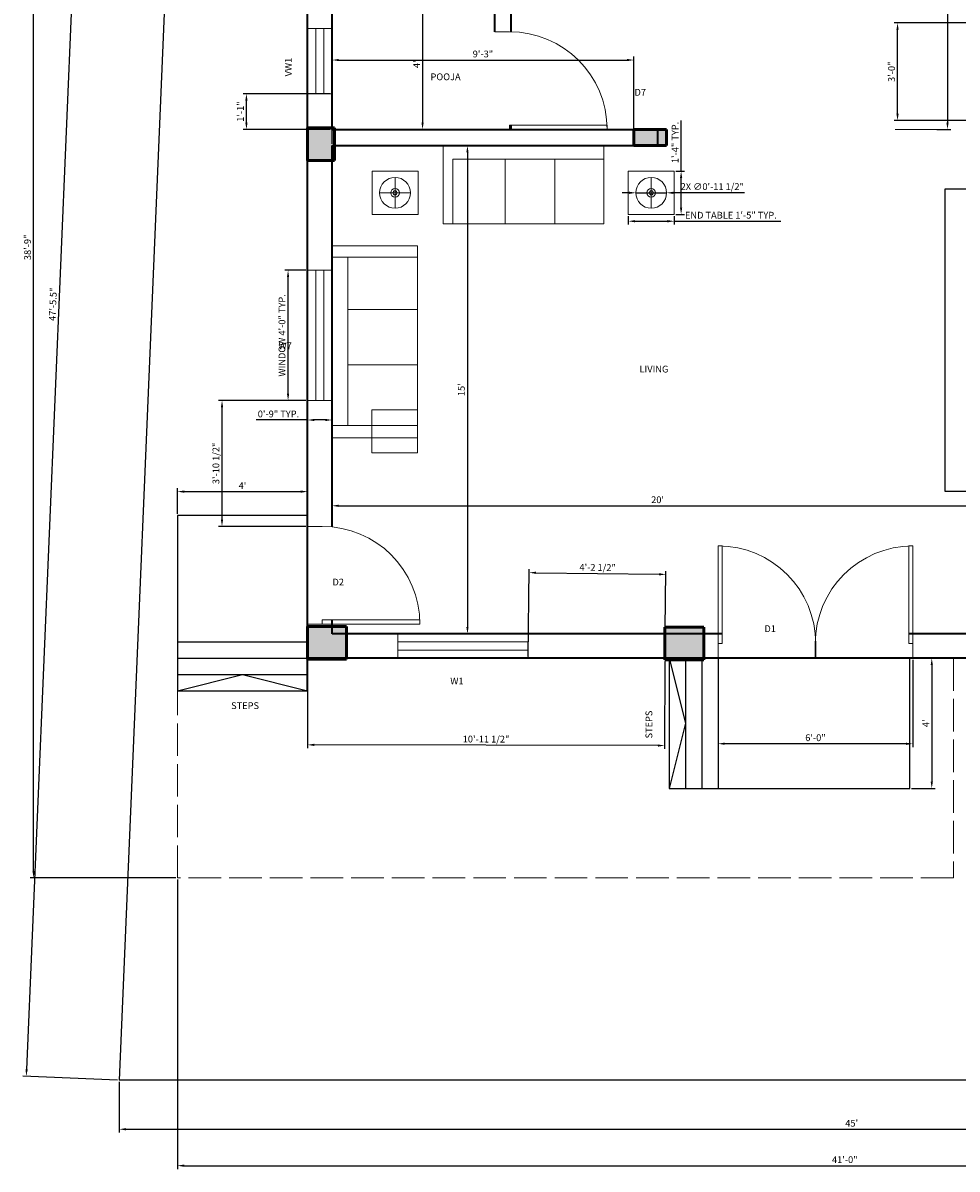
# Model space of a CAD drawing. Units: inches. Extents: x 2470 to 6338, y 1562 to 4199.
# Tile 1 of 5: x 2471 to 2816, y 1562 to 1985. Entities that reach past the tile are written whole.
import ezdxf

# ---------------------------------------------------------------- set-up
doc = ezdxf.new("R2010")
doc.units = ezdxf.units.IN
doc.linetypes.add('ACAD_ISO02W100', pattern=[15, 12, -3])
for name, color, linetype, lineweight in [('A-ANNO-DIMS', 2, 'Continuous', 18), ('A-ANNO-TEXT', 7, 'Continuous', 18), ('A-AREA-IDEN', 7, 'Continuous', 25), ('A-COLS', 1, 'Continuous', 50), ('A-DOOR', 4, 'Continuous', 18), ('A-FLOR-OVHD', 8, 'ACAD_ISO02W100', 18), ('A-FLOR-STRS', 7, 'Continuous', 25), ('A-FURN', 8, 'Continuous', 18), ('A-FURN-FIXD', 8, 'Continuous', 25), ('A-GLAZ', 4, 'Continuous', 18), ('A-WALL', 7, 'Continuous', 35), ('C-PROP', 3, 'Continuous', 25)]:
    doc.layers.add(name, color=color, linetype=linetype, lineweight=lineweight)
doc.styles.get("Standard").update_dxf_attribs({"font": 'arial.ttf'})
doc.dimstyles.new('ISO-25', dxfattribs={"dimtxt": 2.5, "dimasz": 2.5, "dimexe": 1.25, "dimexo": 0.625, "dimtad": 1, "dimdec": 1, "dimlunit": 3, "dimtxsty": 'Standard', "dimcen": 2.5, "dimadec": 0, "dimazin": 0, "dimtfac": 1, "dimtdec": 1, "dimtmove": 0, "dimatfit": 3, "dimfxl": 1, "dimarcsym": 0})

# ---------------------------------------------------------------- blocks, each defined once
blk = doc.blocks.new('*U2')
for p, q in [((0, 0), (0, -6)), ((40, 0), (40, -6))]:
    blk.add_line(p, q)
blk.add_lwpolyline([(0, 0), (0, 40), (1.75, 40), (1.75, 0)], close=True)
blk.add_arc((0, 0), 40, 0, 90)
blk = doc.blocks.new('*D7')
at = {"layer": 'A-ANNO-DIMS', "color": 0, "lineweight": -2, "transparency": 16777216}
for p, q in [((2530.1, 2164.02), (2495.24, 2165.49)), ((2496.38, 2162.94), (2472.59, 1598.93)), ((2506.1, 1595.02), (2471.24, 1596.49))]:
    blk.add_line(p, q, dxfattribs=at)
at = {"layer": 'A-ANNO-DIMS', "color": 0, "lineweight": 100, "transparency": 16777216}
for points in [[(2495.96, 2162.95), (2496.8, 2162.92), (2496.48, 2165.43)], [(2472.17, 1598.95), (2473.01, 1598.92), (2472.48, 1596.43)]]:
    blk.add_solid(points, dxfattribs=at)
at = {"layer": 'Defpoints', "color": 0, "lineweight": 100, "transparency": 16777216}
for p in [(2530.72, 2163.99), (2472.48, 1596.43), (2506.72, 1594.99)]:
    blk.add_point(p, dxfattribs=at)
at = {"layer": 'A-ANNO-DIMS', "color": 0, "transparency": 16777216, "insert": (2482.59, 1881.01), "char_height": 2.5, "attachment_point": 5, "rotation": 87.5847}
blk.add_mtext('47\'-5.5"', dxfattribs=at)
blk = doc.blocks.new('*D10')
at = {"layer": 'A-ANNO-DIMS', "color": 0, "lineweight": -2, "transparency": 16777216}
for p, q in [((2506.72, 1594.37), (2506.72, 1575.62)), ((3046.72, 1594.37), (3046.72, 1575.62)), ((2509.22, 1576.87), (3044.22, 1576.87))]:
    blk.add_line(p, q, dxfattribs=at)
at = {"layer": 'A-ANNO-DIMS', "color": 0, "lineweight": 100, "transparency": 16777216}
for points in [[(2509.22, 1577.29), (2509.22, 1576.46), (2506.72, 1576.87)], [(3044.22, 1577.29), (3044.22, 1576.46), (3046.72, 1576.87)]]:
    blk.add_solid(points, dxfattribs=at)
at = {"layer": 'Defpoints', "color": 0, "lineweight": 100, "transparency": 16777216}
for p in [(2506.72, 1594.99), (3046.72, 1594.99), (3046.72, 1576.87)]:
    blk.add_point(p, dxfattribs=at)
at = {"layer": 'A-ANNO-DIMS', "color": 0, "transparency": 16777216, "insert": (2776.72, 1578.77), "char_height": 2.5, "attachment_point": 5}
blk.add_mtext("45'", dxfattribs=at)
blk = doc.blocks.new('*D13')
at = {"layer": 'A-ANNO-DIMS', "color": 0, "lineweight": -2, "transparency": 16777216}
for p, q in [((2528.17, 1803.76), (2528.17, 1813.21)), ((2576.17, 1803.76), (2576.17, 1813.21)), ((2530.67, 1811.96), (2573.67, 1811.96))]:
    blk.add_line(p, q, dxfattribs=at)
at = {"layer": 'A-ANNO-DIMS', "color": 0, "lineweight": 100, "transparency": 16777216}
for points in [[(2530.67, 1812.38), (2530.67, 1811.55), (2528.17, 1811.96)], [(2573.67, 1812.38), (2573.67, 1811.55), (2576.17, 1811.96)]]:
    blk.add_solid(points, dxfattribs=at)
at = {"layer": 'Defpoints', "color": 0, "lineweight": 100, "transparency": 16777216}
for p in [(2576.17, 1811.96), (2528.17, 1803.13), (2576.17, 1803.13)]:
    blk.add_point(p, dxfattribs=at)
at = {"layer": 'A-ANNO-DIMS', "color": 0, "transparency": 16777216, "insert": (2552.17, 1813.84), "char_height": 2.5, "attachment_point": 5}
blk.add_mtext("4'", dxfattribs=at)
blk = doc.blocks.new('*D14')
at = {"layer": 'A-ANNO-DIMS', "color": 0, "lineweight": -2, "transparency": 16777216}
for p, q in [((2798.79, 1750.53), (2807.48, 1750.53)), ((2806.23, 1748.03), (2806.23, 1705.06)), ((2798.79, 1702.56), (2807.48, 1702.56))]:
    blk.add_line(p, q, dxfattribs=at)
at = {"layer": 'A-ANNO-DIMS', "color": 0, "lineweight": 100, "transparency": 16777216}
for points in [[(2805.82, 1748.03), (2806.65, 1748.03), (2806.23, 1750.53)], [(2805.82, 1705.06), (2806.65, 1705.06), (2806.23, 1702.56)]]:
    blk.add_solid(points, dxfattribs=at)
at = {"layer": 'Defpoints', "color": 0, "lineweight": 100, "transparency": 16777216}
for p in [(2798.17, 1750.53), (2798.17, 1702.56), (2806.23, 1702.56)]:
    blk.add_point(p, dxfattribs=at)
at = {"layer": 'A-ANNO-DIMS', "color": 0, "transparency": 16777216, "insert": (2804.36, 1726.55), "char_height": 2.5, "attachment_point": 5, "rotation": 90}
blk.add_mtext("4'", dxfattribs=at)
blk = doc.blocks.new('*D15')
at = {"layer": 'A-ANNO-DIMS', "color": 0, "lineweight": -2, "transparency": 16777216}
for p, q in [((2585.17, 1813.52), (2585.17, 1805.49)), ((2825.17, 1813.52), (2825.17, 1805.49)), ((2587.67, 1806.74), (2822.67, 1806.74))]:
    blk.add_line(p, q, dxfattribs=at)
at = {"layer": 'A-ANNO-DIMS', "color": 0, "lineweight": 100, "transparency": 16777216}
for points in [[(2587.67, 1807.16), (2587.67, 1806.32), (2585.17, 1806.74)], [(2822.67, 1807.16), (2822.67, 1806.32), (2825.17, 1806.74)]]:
    blk.add_solid(points, dxfattribs=at)
at = {"layer": 'Defpoints', "color": 0, "lineweight": 100, "transparency": 16777216}
for p in [(2585.17, 1814.14), (2825.17, 1814.14), (2825.17, 1806.74)]:
    blk.add_point(p, dxfattribs=at)
at = {"layer": 'A-ANNO-DIMS', "color": 0, "transparency": 16777216, "insert": (2705.17, 1808.64), "char_height": 2.5, "attachment_point": 5}
blk.add_mtext("20'", dxfattribs=at)
blk = doc.blocks.new('*D16')
at = {"layer": 'A-ANNO-DIMS', "color": 0, "lineweight": -2, "transparency": 16777216}
for p, q in [((2621.84, 1939.53), (2636.34, 1939.53)), ((2635.09, 1937.03), (2635.09, 1762.03)), ((2621.84, 1759.53), (2636.34, 1759.53))]:
    blk.add_line(p, q, dxfattribs=at)
at = {"layer": 'A-ANNO-DIMS', "color": 0, "lineweight": 100, "transparency": 16777216}
for points in [[(2634.67, 1937.03), (2635.5, 1937.03), (2635.09, 1939.53)], [(2634.67, 1762.03), (2635.5, 1762.03), (2635.09, 1759.53)]]:
    blk.add_solid(points, dxfattribs=at)
at = {"layer": 'Defpoints', "color": 0, "lineweight": 100, "transparency": 16777216}
for p in [(2621.21, 1939.53), (2621.21, 1759.53), (2635.09, 1759.53)]:
    blk.add_point(p, dxfattribs=at)
at = {"layer": 'A-ANNO-DIMS', "color": 0, "transparency": 16777216, "insert": (2633.18, 1849.53), "char_height": 2.5, "attachment_point": 5, "rotation": 90}
blk.add_mtext("15'", dxfattribs=at)
blk = doc.blocks.new('*D23')
at = {"layer": 'A-ANNO-DIMS', "color": 0, "lineweight": -2, "transparency": 16777216}
for p, q in [((2615.79, 1993.53), (2619.79, 1993.53)), ((2618.54, 1991.03), (2618.54, 1948.03)), ((2615.79, 1945.53), (2619.79, 1945.53))]:
    blk.add_line(p, q, dxfattribs=at)
at = {"layer": 'A-ANNO-DIMS', "color": 0, "lineweight": 100, "transparency": 16777216}
for points in [[(2618.13, 1991.03), (2618.96, 1991.03), (2618.54, 1993.53)], [(2618.13, 1948.03), (2618.96, 1948.03), (2618.54, 1945.53)]]:
    blk.add_solid(points, dxfattribs=at)
at = {"layer": 'Defpoints', "color": 0, "lineweight": 100, "transparency": 16777216}
for p in [(2615.17, 1993.53), (2615.17, 1945.53), (2618.54, 1945.53)]:
    blk.add_point(p, dxfattribs=at)
at = {"layer": 'A-ANNO-DIMS', "color": 0, "transparency": 16777216, "insert": (2616.67, 1969.53), "char_height": 2.5, "attachment_point": 5, "rotation": 90}
blk.add_mtext("4'", dxfattribs=at)
blk = doc.blocks.new('*D28')
at = {"layer": 'A-ANNO-DIMS', "color": 0, "lineweight": -2, "transparency": 16777216}
for p, q in [((2808.15, 2125.53), (2813.28, 2125.53)), ((2812.03, 2123.03), (2812.03, 1948.03)), ((2808.15, 1945.53), (2813.28, 1945.53))]:
    blk.add_line(p, q, dxfattribs=at)
at = {"layer": 'A-ANNO-DIMS', "color": 0, "lineweight": 100, "transparency": 16777216}
for points in [[(2811.62, 2123.03), (2812.45, 2123.03), (2812.03, 2125.53)], [(2811.62, 1948.03), (2812.45, 1948.03), (2812.03, 1945.53)]]:
    blk.add_solid(points, dxfattribs=at)
at = {"layer": 'Defpoints', "color": 0, "lineweight": 100, "transparency": 16777216}
for p in [(2807.53, 2125.53), (2807.53, 1945.53), (2812.03, 1945.53)]:
    blk.add_point(p, dxfattribs=at)
at = {"layer": 'A-ANNO-DIMS', "color": 0, "transparency": 16777216, "insert": (2810.13, 2035.53), "char_height": 2.5, "attachment_point": 5, "rotation": 90}
blk.add_mtext("15'", dxfattribs=at)
blk = doc.blocks.new('WIN-48IN')
for p, q in [((0, 9), (48, 9)), ((0, 0), (0, 9)), ((48, 9), (48, 0)), ((0, 6), (48, 6)), ((48, 3), (0, 3)), ((48, 0), (0, 0))]:
    blk.add_line(p, q)
blk = doc.blocks.new('VENT-WIN-24IN')
for p, q in [((9, 24), (0, 24)), ((0, 24), (0, 0)), ((3, 24), (3, 0)), ((6, 0), (6, 24)), ((9, 0), (9, 24)), ((0, 0), (9, 0))]:
    blk.add_line(p, q)
blk = doc.blocks.new('COL-6X12')
h = blk.add_hatch(color=256)
h.dxf.hatch_style = 1
h.paths.add_polyline_path([(6, 12), (0, 12), (0, 0), (6, 0)])
for p, q in [((6, 12), (0, 12)), ((0, 12), (0, 0)), ((6, 0), (6, 12)), ((0, 0), (6, 0))]:
    blk.add_line(p, q)
blk = doc.blocks.new('COL-10X12')
h = blk.add_hatch(color=256)
h.dxf.hatch_style = 1
h.paths.add_polyline_path([(10, 12), (0, 12), (0, 0), (10, 0)])
for p, q in [((10, 12), (0, 12)), ((0, 12), (0, 0)), ((10, 0), (10, 12)), ((0, 0), (10, 0))]:
    blk.add_line(p, q)
blk = doc.blocks.new('COL-RECT-LARGE')
h = blk.add_hatch(color=256)
h.dxf.hatch_style = 1
h.paths.add_polyline_path([(14.33, 12.11), (10, 12.11), (0, 12.11), (0, 0), (10, 0), (14.33, 0)])
for p, q in [((10, 12.11), (0, 12.11)), ((0, 12.11), (0, 0)), ((10, 12.11), (14.33, 12.11)), ((14.33, 12.11), (14.33, 0)), ((10, 0), (0, 0)), ((14.33, 0), (10, 0))]:
    blk.add_line(p, q)
blk = doc.blocks.new('END-TABLE-LAMP')
for q in [(8.47, 13.6), (2.8, 7.93), (14.14, 7.93), (8.47, 2.26)]:
    blk.add_line((8.47, 7.93), q)
blk.add_lwpolyline([(0, 15.87), (16.95, 15.87), (16.95, 0), (0, 0)], close=True)
for radius in [5.67, 1.6, 0.75]:
    blk.add_circle((8.47, 7.93), radius)
blk = doc.blocks.new('*D38')
at = {"layer": 'A-ANNO-DIMS', "color": 0, "lineweight": -2, "transparency": 16777216}
for p, q in [((2575.54, 1893.57), (2567.72, 1893.57)), ((2568.97, 1848.07), (2568.97, 1891.07)), ((2575.54, 1845.57), (2567.72, 1845.57))]:
    blk.add_line(p, q, dxfattribs=at)
at = {"layer": 'A-ANNO-DIMS', "color": 0, "lineweight": 100, "transparency": 16777216}
for points in [[(2568.55, 1891.07), (2569.38, 1891.07), (2568.97, 1893.57)], [(2568.55, 1848.07), (2569.38, 1848.07), (2568.97, 1845.57)]]:
    blk.add_solid(points, dxfattribs=at)
at = {"layer": 'Defpoints', "color": 0, "lineweight": 100, "transparency": 16777216}
for p in [(2568.97, 1893.57), (2576.17, 1893.57), (2576.17, 1845.57)]:
    blk.add_point(p, dxfattribs=at)
at = {"layer": 'A-ANNO-DIMS', "color": 0, "transparency": 16777216, "insert": (2567.05, 1869.57), "char_height": 2.5, "attachment_point": 5, "rotation": 90}
blk.add_mtext('WINDOW 4\'-0" TYP.', dxfattribs=at)
blk = doc.blocks.new('*D39')
at = {"layer": 'A-ANNO-DIMS', "color": 0, "lineweight": -2, "transparency": 16777216}
for p, q in [((2576.17, 1844.94), (2576.17, 1837.12)), ((2585.17, 1844.94), (2585.17, 1837.12)), ((2576.17, 1838.37), (2557.18, 1838.37)), ((2582.67, 1838.37), (2578.67, 1838.37))]:
    blk.add_line(p, q, dxfattribs=at)
at = {"layer": 'A-ANNO-DIMS', "color": 0, "lineweight": 100, "transparency": 16777216}
for points in [[(2578.67, 1838.79), (2578.67, 1837.95), (2576.17, 1838.37)], [(2582.67, 1838.79), (2582.67, 1837.95), (2585.17, 1838.37)]]:
    blk.add_solid(points, dxfattribs=at)
at = {"layer": 'Defpoints', "color": 0, "lineweight": 100, "transparency": 16777216}
for p in [(2576.17, 1845.57), (2585.17, 1845.57), (2576.17, 1838.37)]:
    blk.add_point(p, dxfattribs=at)
at = {"layer": 'A-ANNO-DIMS', "color": 0, "transparency": 16777216, "insert": (2565.42, 1840.27), "char_height": 2.5, "attachment_point": 5}
blk.add_mtext('0\'-9" TYP.', dxfattribs=at)
blk = doc.blocks.new('*D50')
at = {"layer": 'A-ANNO-DIMS', "color": 0, "lineweight": -2, "transparency": 16777216}
for p, q in [((2694.36, 1913.57), (2694.36, 1910.4)), ((2696.86, 1911.65), (2708.8, 1911.65)), ((2711.3, 1913.57), (2711.3, 1910.4)), ((2711.3, 1911.65), (2750.54, 1911.65))]:
    blk.add_line(p, q, dxfattribs=at)
at = {"layer": 'A-ANNO-DIMS', "color": 0, "lineweight": 100, "transparency": 16777216}
for points in [[(2696.86, 1912.07), (2696.86, 1911.23), (2694.36, 1911.65)], [(2708.8, 1912.07), (2708.8, 1911.23), (2711.3, 1911.65)]]:
    blk.add_solid(points, dxfattribs=at)
at = {"layer": 'Defpoints', "color": 0, "lineweight": 100, "transparency": 16777216}
for p in [(2694.36, 1914.19), (2711.3, 1914.19), (2711.3, 1911.65)]:
    blk.add_point(p, dxfattribs=at)
at = {"layer": 'A-ANNO-DIMS', "color": 0, "transparency": 16777216, "insert": (2732.17, 1913.55), "char_height": 2.5, "attachment_point": 5}
blk.add_mtext('END TABLE 1\'-5" TYP.', dxfattribs=at)
blk = doc.blocks.new('*D51')
at = {"layer": 'A-ANNO-DIMS', "color": 0, "lineweight": -2, "transparency": 16777216}
for p, q in [((2713.84, 1930.06), (2713.84, 1948.81)), ((2711.93, 1930.06), (2715.09, 1930.06)), ((2713.84, 1916.69), (2713.84, 1927.56)), ((2711.93, 1914.19), (2715.09, 1914.19))]:
    blk.add_line(p, q, dxfattribs=at)
at = {"layer": 'A-ANNO-DIMS', "color": 0, "lineweight": 100, "transparency": 16777216}
for points in [[(2713.43, 1927.56), (2714.26, 1927.56), (2713.84, 1930.06)], [(2713.43, 1916.69), (2714.26, 1916.69), (2713.84, 1914.19)]]:
    blk.add_solid(points, dxfattribs=at)
at = {"layer": 'Defpoints', "color": 0, "lineweight": 100, "transparency": 16777216}
for p in [(2711.3, 1930.06), (2713.84, 1930.06), (2711.3, 1914.19)]:
    blk.add_point(p, dxfattribs=at)
at = {"layer": 'A-ANNO-DIMS', "color": 0, "transparency": 16777216, "insert": (2711.96, 1940.69), "char_height": 2.5, "attachment_point": 5, "rotation": 90}
blk.add_mtext('1\'-4" TYP.', dxfattribs=at)
blk = doc.blocks.new('*D58')
at = {"layer": 'A-ANNO-DIMS', "color": 0, "lineweight": -2, "transparency": 16777216}
for p, q in [((3020.17, 1673.39), (3020.17, 1562.19)), ((2528.17, 1668.91), (2528.17, 1562.19)), ((2530.67, 1563.44), (3017.67, 1563.44))]:
    blk.add_line(p, q, dxfattribs=at)
at = {"layer": 'A-ANNO-DIMS', "color": 0, "lineweight": 100, "transparency": 16777216}
for points in [[(2530.67, 1563.86), (2530.67, 1563.02), (2528.17, 1563.44)], [(3017.67, 1563.86), (3017.67, 1563.02), (3020.17, 1563.44)]]:
    blk.add_solid(points, dxfattribs=at)
at = {"layer": 'Defpoints', "color": 0, "lineweight": 100, "transparency": 16777216}
for p in [(3020.17, 1674.02), (2528.17, 1669.53), (3020.17, 1563.44)]:
    blk.add_point(p, dxfattribs=at)
at = {"layer": 'A-ANNO-DIMS', "color": 0, "transparency": 16777216, "insert": (2774.17, 1565.34), "char_height": 2.5, "attachment_point": 5}
blk.add_mtext('41\'-0"', dxfattribs=at)
blk = doc.blocks.new('*D59')
at = {"layer": 'A-ANNO-DIMS', "color": 0, "lineweight": -2, "transparency": 16777216}
for p, q in [((2575.54, 2134.53), (2473.92, 2134.53)), ((2475.17, 1672.03), (2475.17, 2132.03)), ((2527.54, 1669.53), (2473.92, 1669.53))]:
    blk.add_line(p, q, dxfattribs=at)
at = {"layer": 'A-ANNO-DIMS', "color": 0, "lineweight": 100, "transparency": 16777216}
for points in [[(2474.76, 2132.03), (2475.59, 2132.03), (2475.17, 2134.53)], [(2474.76, 1672.03), (2475.59, 1672.03), (2475.17, 1669.53)]]:
    blk.add_solid(points, dxfattribs=at)
at = {"layer": 'Defpoints', "color": 0, "lineweight": 100, "transparency": 16777216}
for p in [(2475.17, 2134.53), (2576.17, 2134.53), (2528.17, 1669.53)]:
    blk.add_point(p, dxfattribs=at)
at = {"layer": 'A-ANNO-DIMS', "color": 0, "transparency": 16777216, "insert": (2473.27, 1902.03), "char_height": 2.5, "attachment_point": 5, "rotation": 90}
blk.add_mtext('38\'-9"', dxfattribs=at)
blk = doc.blocks.new('*D62')
at = {"layer": 'A-ANNO-DIMS', "color": 0, "lineweight": -2, "transparency": 16777216}
for p, q in [((2576.17, 1749.52), (2576.1, 1717.35)), ((2707.83, 1749.27), (2707.77, 1717.09)), ((2705.27, 1718.35), (2578.61, 1718.59))]:
    blk.add_line(p, q, dxfattribs=at)
at = {"layer": 'A-ANNO-DIMS', "color": 0, "lineweight": 100, "transparency": 16777216}
for points in [[(2578.61, 1719.01), (2578.61, 1718.18), (2576.11, 1718.6)], [(2705.27, 1718.76), (2705.27, 1717.93), (2707.77, 1718.34)]]:
    blk.add_solid(points, dxfattribs=at)
at = {"layer": 'Defpoints', "color": 0, "lineweight": 100, "transparency": 16777216}
for p in [(2576.17, 1750.15), (2707.83, 1749.89), (2576.11, 1718.6)]:
    blk.add_point(p, dxfattribs=at)
at = {"layer": 'A-ANNO-DIMS', "color": 0, "transparency": 16777216, "insert": (2641.94, 1720.39), "char_height": 2.5, "attachment_point": 5, "rotation": 359.8882}
blk.add_mtext('10\'-11 1/2"', dxfattribs=at)
blk = doc.blocks.new('*D65')
at = {"layer": 'A-ANNO-DIMS', "color": 0, "lineweight": -2, "transparency": 16777216}
for p, q in [((2585.17, 1940.16), (2585.17, 1972.33)), ((2587.67, 1971.08), (2693.91, 1971.08)), ((2696.41, 1940.16), (2696.41, 1972.33))]:
    blk.add_line(p, q, dxfattribs=at)
at = {"layer": 'A-ANNO-DIMS', "color": 0, "lineweight": 100, "transparency": 16777216}
for points in [[(2587.67, 1971.5), (2587.67, 1970.67), (2585.17, 1971.08)], [(2693.91, 1971.5), (2693.91, 1970.67), (2696.41, 1971.08)]]:
    blk.add_solid(points, dxfattribs=at)
at = {"layer": 'Defpoints', "color": 0, "lineweight": 100, "transparency": 16777216}
for p in [(2696.41, 1971.08), (2585.17, 1939.53), (2696.41, 1939.53)]:
    blk.add_point(p, dxfattribs=at)
at = {"layer": 'A-ANNO-DIMS', "color": 0, "transparency": 16777216, "insert": (2640.79, 1972.99), "char_height": 2.5, "attachment_point": 5}
blk.add_mtext('9\'-3"', dxfattribs=at)
blk = doc.blocks.new('*D68')
at = {"layer": 'A-ANNO-DIMS', "color": 0, "lineweight": -2, "transparency": 16777216}
for p, q in [((2727.46, 1749.94), (2727.44, 1717.76)), ((2799.3, 1749.91), (2799.29, 1717.73)), ((2796.79, 1718.99), (2729.94, 1719.01))]:
    blk.add_line(p, q, dxfattribs=at)
at = {"layer": 'A-ANNO-DIMS', "color": 0, "lineweight": 100, "transparency": 16777216}
for points in [[(2729.94, 1719.43), (2729.94, 1718.59), (2727.44, 1719.01)], [(2796.79, 1719.4), (2796.79, 1718.57), (2799.29, 1718.98)]]:
    blk.add_solid(points, dxfattribs=at)
at = {"layer": 'Defpoints', "color": 0, "lineweight": 100, "transparency": 16777216}
for p in [(2727.46, 1750.56), (2799.3, 1750.53), (2727.44, 1719.01)]:
    blk.add_point(p, dxfattribs=at)
at = {"layer": 'A-ANNO-DIMS', "color": 0, "transparency": 16777216, "insert": (2763.37, 1720.9), "char_height": 2.5, "attachment_point": 5, "rotation": 359.9793}
blk.add_mtext('6\'-0"', dxfattribs=at)
blk = doc.blocks.new('*D69')
at = {"layer": 'A-ANNO-DIMS', "color": 0, "lineweight": -2, "transparency": 16777216}
for p, q in [((2824.54, 1984.76), (2792.37, 1984.76)), ((2793.62, 1951.26), (2793.62, 1982.26)), ((2824.54, 1948.76), (2792.37, 1948.76))]:
    blk.add_line(p, q, dxfattribs=at)
at = {"layer": 'A-ANNO-DIMS', "color": 0, "lineweight": 100, "transparency": 16777216}
for points in [[(2793.2, 1982.26), (2794.03, 1982.26), (2793.62, 1984.76)], [(2793.2, 1951.26), (2794.03, 1951.26), (2793.62, 1948.76)]]:
    blk.add_solid(points, dxfattribs=at)
at = {"layer": 'Defpoints', "color": 0, "lineweight": 100, "transparency": 16777216}
for p in [(2793.62, 1984.76), (2825.17, 1984.76), (2825.17, 1948.76)]:
    blk.add_point(p, dxfattribs=at)
at = {"layer": 'A-ANNO-DIMS', "color": 0, "transparency": 16777216, "insert": (2791.72, 1966.76), "char_height": 2.5, "attachment_point": 5, "rotation": 90}
blk.add_mtext('3\'-0"', dxfattribs=at)
blk = doc.blocks.new('*D73')
at = {"layer": 'A-ANNO-DIMS', "color": 0, "lineweight": -2, "transparency": 16777216}
for p, q in [((2657.46, 1751.16), (2657.87, 1783.33)), ((2660.35, 1782.05), (2705.73, 1781.47)), ((2707.84, 1750.52), (2708.25, 1782.69))]:
    blk.add_line(p, q, dxfattribs=at)
at = {"layer": 'A-ANNO-DIMS', "color": 0, "lineweight": 100, "transparency": 16777216}
for points in [[(2660.36, 1782.47), (2660.35, 1781.63), (2657.85, 1782.08)], [(2705.74, 1781.89), (2705.73, 1781.05), (2708.23, 1781.44)]]:
    blk.add_solid(points, dxfattribs=at)
at = {"layer": 'Defpoints', "color": 0, "lineweight": 100, "transparency": 16777216}
for p in [(2708.23, 1781.44), (2657.45, 1750.53), (2707.83, 1749.89)]:
    blk.add_point(p, dxfattribs=at)
at = {"layer": 'A-ANNO-DIMS', "color": 0, "transparency": 16777216, "insert": (2683.07, 1783.68), "char_height": 2.5, "attachment_point": 5, "rotation": 359.2699}
blk.add_mtext('4\'-2 1/2"', dxfattribs=at)
blk = doc.blocks.new('*D75')
at = {"layer": 'A-ANNO-DIMS', "color": 0, "lineweight": -2, "transparency": 16777216}
for p, q in [((2575.54, 1845.57), (2543.37, 1845.57)), ((2544.62, 1801.65), (2544.62, 1843.07)), ((2575.54, 1799.15), (2543.37, 1799.15))]:
    blk.add_line(p, q, dxfattribs=at)
at = {"layer": 'A-ANNO-DIMS', "color": 0, "lineweight": 100, "transparency": 16777216}
for points in [[(2544.2, 1843.07), (2545.03, 1843.07), (2544.62, 1845.57)], [(2544.2, 1801.65), (2545.03, 1801.65), (2544.62, 1799.15)]]:
    blk.add_solid(points, dxfattribs=at)
at = {"layer": 'Defpoints', "color": 0, "lineweight": 100, "transparency": 16777216}
for p in [(2544.62, 1845.57), (2576.17, 1845.57), (2576.17, 1799.15)]:
    blk.add_point(p, dxfattribs=at)
at = {"layer": 'A-ANNO-DIMS', "color": 0, "transparency": 16777216, "insert": (2542.7, 1822.36), "char_height": 2.5, "attachment_point": 5, "rotation": 90}
blk.add_mtext('3\'-10 1/2"', dxfattribs=at)
blk = doc.blocks.new('*D77')
at = {"layer": 'A-ANNO-DIMS', "color": 0, "lineweight": -2, "transparency": 16777216}
for p, q in [((2584.54, 1958.65), (2552.37, 1958.65)), ((2553.62, 1948.03), (2553.62, 1956.15)), ((2584.54, 1945.53), (2552.37, 1945.53))]:
    blk.add_line(p, q, dxfattribs=at)
at = {"layer": 'A-ANNO-DIMS', "color": 0, "lineweight": 100, "transparency": 16777216}
for points in [[(2553.2, 1956.15), (2554.03, 1956.15), (2553.62, 1958.65)], [(2553.2, 1948.03), (2554.03, 1948.03), (2553.62, 1945.53)]]:
    blk.add_solid(points, dxfattribs=at)
at = {"layer": 'Defpoints', "color": 0, "lineweight": 100, "transparency": 16777216}
for p in [(2553.62, 1958.65), (2585.17, 1958.65), (2585.17, 1945.53)]:
    blk.add_point(p, dxfattribs=at)
at = {"layer": 'A-ANNO-DIMS', "color": 0, "transparency": 16777216, "insert": (2551.74, 1952.09), "char_height": 2.5, "attachment_point": 5, "rotation": 90}
blk.add_mtext('1\'-1"', dxfattribs=at)
blk = doc.blocks.new('*D82')
at = {"layer": 'A-ANNO-DIMS', "color": 0, "lineweight": -2, "transparency": 16777216}
for p, q in [((2694.66, 1922.13), (2692.16, 1922.13)), ((2697.16, 1922.13), (2708.5, 1922.13)), ((2737.16, 1922.13), (2711, 1922.13))]:
    blk.add_line(p, q, dxfattribs=at)
at = {"layer": 'A-ANNO-DIMS', "color": 0, "lineweight": 100, "transparency": 16777216}
for points in [[(2694.66, 1922.54), (2694.66, 1921.71), (2697.16, 1922.13)], [(2711, 1922.54), (2711, 1921.71), (2708.5, 1922.13)]]:
    blk.add_solid(points, dxfattribs=at)
at = {"layer": 'Defpoints', "color": 0, "lineweight": 100, "transparency": 16777216}
for p in [(2697.16, 1922.13), (2708.5, 1922.13)]:
    blk.add_point(p, dxfattribs=at)
at = {"layer": 'A-ANNO-DIMS', "color": 0, "transparency": 16777216, "insert": (2725.33, 1924.1), "char_height": 2.5, "attachment_point": 5, "rotation": 0.0015}
blk.add_mtext('2X ∅0\'-11 1/2"', dxfattribs=at)

msp = doc.modelspace()

# ---------------------------------------------------------------- linework, layer by layer
at = {"layer": 'A-ANNO-DIMS'}
msp.add_line((2812.91, 1945.53), (2792.69, 1945.53), dxfattribs=at)
at = {"layer": 'A-FLOR-OVHD'}
for p, q in [((2528.17, 1669.53), (2528.17, 1803.13)), ((2814.26, 1750.53), (2814.26, 1669.53)), ((2814.26, 1669.53), (2528.17, 1669.53))]:
    msp.add_line(p, q, dxfattribs=at)
at = {"layer": 'A-FLOR-STRS'}
for p, q in [((2576.17, 1803.13), (2528.17, 1803.13)), ((2528.17, 1803.13), (2528.17, 1738.53)), ((2528.17, 1756.53), (2576.17, 1756.53)), ((2528.17, 1750.53), (2576.17, 1750.53)), ((2709.46, 1750.56), (2709.46, 1702.56)), ((2709.46, 1750.56), (2715.46, 1726.56)), ((2715.46, 1750.56), (2715.46, 1702.56)), ((2721.46, 1750.56), (2721.46, 1702.56)), ((2727.46, 1750.56), (2727.46, 1702.56)), ((2798.17, 1702.56), (2798.17, 1750.56)), ((2528.17, 1744.53), (2576.17, 1744.53)), ((2528.17, 1738.53), (2552.17, 1744.53)), ((2552.17, 1744.53), (2576.17, 1738.53)), ((2528.17, 1738.53), (2576.17, 1738.53)), ((2715.46, 1726.56), (2709.46, 1702.56)), ((2709.46, 1702.56), (2798.17, 1702.56))]:
    msp.add_line(p, q, dxfattribs=at)
at = {"layer": 'A-FURN'}
for p, q in [((2629.73, 1910.73), (2629.73, 1934.55)), ((2629.73, 1934.55), (2685.39, 1934.55)), ((2648.97, 1934.55), (2648.97, 1910.73)), ((2667.26, 1934.55), (2667.26, 1910.73)), ((2585.17, 1902.57), (2616.68, 1902.57)), ((2616.68, 1902.57), (2616.68, 1898.45)), ((2590.97, 1898.45), (2590.97, 1836.38)), ((2590.97, 1879.12), (2616.68, 1879.12)), ((2590.97, 1858.66), (2616.68, 1858.66)), ((2616.68, 1836.38), (2616.68, 1831.83)), ((2616.68, 1831.83), (2585.17, 1831.83))]:
    msp.add_line(p, q, dxfattribs=at)
for points in [[(2626.15, 1939.53), (2685.39, 1939.53), (2685.39, 1910.73), (2626.15, 1910.73)], [(2585.17, 1898.45), (2616.68, 1898.45), (2616.68, 1836.38), (2585.17, 1836.38)], [(2616.68, 1842.11), (2599.9, 1842.11), (2599.9, 1826.2), (2616.68, 1826.2)]]:
    msp.add_lwpolyline(points, close=True, dxfattribs=at)
at = {"layer": 'A-FURN-FIXD'}
msp.add_lwpolyline([(2825.17, 1923.49), (2811.05, 1923.49), (2811.05, 1812.14), (2825.17, 1812.14)], close=True, dxfattribs=at)
at = {"layer": 'A-WALL'}
for p, q in [((2576.17, 1763.15), (2576.17, 2134.53)), ((2651.17, 1981.53), (2651.17, 1999.53)), ((2585.17, 1945.53), (2585.17, 1993.53)), ((2645.17, 1981.53), (2645.17, 1993.53)), ((2585.17, 1945.53), (2705.17, 1945.53)), ((2651.17, 1945.53), (2651.17, 1947.11)), ((2705.17, 1945.53), (2705.17, 1939.53)), ((2585.17, 1939.53), (2705.17, 1939.53)), ((2585.17, 1798.97), (2585.17, 1939.53)), ((2576.17, 1738.53), (2576.17, 1763.15)), ((2585.17, 1759.53), (2585.17, 1764.72)), ((2729.03, 1759.53), (2585.17, 1759.53)), ((2763.48, 1759.53), (2763.28, 1759.53)), ((2957.17, 1759.53), (2797.73, 1759.53)), ((3020.17, 1750.53), (2576.17, 1750.53))]:
    msp.add_line(p, q, dxfattribs=at)
at = {"layer": 'C-PROP'}
for p in [(2530.72, 2163.99), (3046.72, 1594.99)]:
    msp.add_line(p, (2506.72, 1594.99), dxfattribs=at)

# ---------------------------------------------------------------- block references
at = {"layer": 'A-COLS'}
for name, p in [('COL-10X12', (2576.1, 1934.05)), ('COL-RECT-LARGE', (2576.17, 1750.15)), ('COL-RECT-LARGE', (2707.83, 1749.89))]:
    msp.add_blockref(name, p, dxfattribs=at)
at = {"layer": 'A-COLS', "extrusion": (0, 0, -1), "zscale": -1, "rotation": 89.99999999999677}
msp.add_blockref('COL-6X12', (-2696.41, 1939.53), dxfattribs=at)
at = {"layer": 'A-DOOR', "xscale": -0.9, "yscale": 0.9, "zscale": 0.9, "rotation": 270}
for p in [(2650.57, 1945.53), (2581.57, 1763.15)]:
    msp.add_blockref('*U2', p, dxfattribs=at)
at = {"layer": 'A-DOOR', "yscale": 0.9, "zscale": 0.9}
for p, xscale in [((2727.46, 1755.96), 0.9), ((2799.3, 1755.93), -0.9)]:
    msp.add_blockref('*U2', p, dxfattribs=dict(at, xscale=xscale))
at = {"layer": 'A-FURN'}
for p in [(2599.92, 1914.19), (2694.36, 1914.19)]:
    msp.add_blockref('END-TABLE-LAMP', p, dxfattribs=at)
at = {"layer": 'A-GLAZ'}
for name, p in [('VENT-WIN-24IN', (2576.17, 1958.65)), ('WIN-48IN', (2609.45, 1750.53))]:
    msp.add_blockref(name, p, dxfattribs=at)
at = {"layer": 'A-GLAZ', "rotation": 90.0000000000017}
msp.add_blockref('WIN-48IN', (2585.17, 1845.57), dxfattribs=at)

# ---------------------------------------------------------------- texts
at = {"layer": 'A-ANNO-TEXT', "char_height": 2.5, "attachment_point": 1, "rotation": 90}
for s, width, insert in [('VW1', 24.2896, (2567.84, 1965.07)), ('STEPS', 18.4844, (2700.72, 1720.95))]:
    msp.add_mtext_dynamic_manual_height_columns(s, width=width, gutter_width=12.5, heights=[0], dxfattribs=dict(at, insert=insert))
at = {"layer": 'A-ANNO-TEXT', "char_height": 2.5, "attachment_point": 1}
for s, width, insert in [('D7', 17.4592, (2696.66, 1960.43)), ('W7', 16.7571, (2565.45, 1866.98)), ('D2', 8.4755, (2585.34, 1779.85)), ('D1', 11.8706, (2744.54, 1762.67)), ('W1', 18.3317, (2628.76, 1743.35)), ('STEPS', 27.3082, (2547.98, 1734.3))]:
    msp.add_mtext_dynamic_manual_height_columns(s, width=width, gutter_width=12.5, heights=[0], dxfattribs=dict(at, insert=insert))
at = {"layer": 'A-AREA-IDEN', "char_height": 2.5, "attachment_point": 1}
for s, width, insert in [('POOJA', 19.9004, (2621.46, 1966.14)), ('LIVING', 61.1706, (2698.51, 1858.38))]:
    msp.add_mtext_dynamic_manual_height_columns(s, width=width, gutter_width=12.5, heights=[0], dxfattribs=dict(at, insert=insert))

# ---------------------------------------------------------------- dimensions: what is measured, and where the dimension line sits
at = {"layer": 'A-ANNO-DIMS'}
dim = msp.add_aligned_dim(p1=(2530.72, 2163.99), p2=(2506.72, 1594.99), distance=-34.27, dimstyle='ISO-25', override={"dimclrd": 0, "dimclre": 0, "dimclrt": 0}, dxfattribs=at)
dim.commit()
dim.dimension.update_dxf_attribs({"geometry": '*D7', "text_midpoint": (2482.59, 1881.01)})
for base, p1, p2, angle, override, picture, middle in [((2475.17, 2134.53), (2528.17, 1669.53), (2576.17, 2134.53), 90, {"dimdec": 1, "dimlfac": 1, "dimrnd": 0, "dimzin": 1, "dimdsep": 46, "dimlunit": 4, "dimfrac": 2}, '*D59', (2473.27, 1902.03)), ((2812.03, 1945.53), (2807.53, 2125.53), (2807.53, 1945.53), 90, {"dimclrd": 0, "dimclre": 0, "dimclrt": 0}, '*D28', (2810.13, 2035.53)), ((2618.54, 1945.53), (2615.17, 1993.53), (2615.17, 1945.53), 90, {"dimclrd": 0, "dimclre": 0, "dimclrt": 0}, '*D23', (2616.67, 1969.53)), ((2793.62, 1984.76), (2825.17, 1948.76), (2825.17, 1984.76), 90, {"dimdec": 1, "dimlfac": 1, "dimrnd": 0, "dimzin": 1, "dimdsep": 46, "dimlunit": 4, "dimfrac": 2}, '*D69', (2791.72, 1966.76)), ((2553.62, 1958.65), (2585.17, 1945.53), (2585.17, 1958.65), 90, {"dimdec": 1, "dimlfac": 1, "dimrnd": 0, "dimzin": 1, "dimdsep": 46, "dimlunit": 4, "dimfrac": 2}, '*D77', (2551.74, 1952.09)), ((2635.09, 1759.53), (2621.21, 1939.53), (2621.21, 1759.53), 90, {"dimclrd": 0, "dimclre": 0, "dimclrt": 0}, '*D16', (2633.18, 1849.53)), ((2544.62, 1845.57), (2576.17, 1799.15), (2576.17, 1845.57), 90, {"dimdec": 1, "dimlfac": 1, "dimrnd": 0, "dimzin": 1, "dimdsep": 46, "dimlunit": 4, "dimfrac": 2}, '*D75', (2542.7, 1822.36)), ((2708.23, 1781.44), (2657.45, 1750.53), (2707.83, 1749.89), 359.2699, {"dimdec": 1, "dimlfac": 1, "dimrnd": 0, "dimzin": 1, "dimdsep": 46, "dimlunit": 4, "dimfrac": 2}, '*D73', (2683.07, 1783.68)), ((2576.11, 1718.6), (2707.83, 1749.89), (2576.17, 1750.15), 179.8882, {"dimdec": 1, "dimlfac": 1, "dimrnd": 0, "dimzin": 1, "dimdsep": 46, "dimlunit": 4, "dimfrac": 2}, '*D62', (2641.94, 1720.39)), ((2727.44, 1719.01), (2799.3, 1750.53), (2727.46, 1750.56), 179.9793, {"dimdec": 1, "dimlfac": 1, "dimrnd": 0, "dimzin": 1, "dimdsep": 46, "dimlunit": 4, "dimfrac": 2}, '*D68', (2763.37, 1720.9)), ((2806.23, 1702.56), (2798.17, 1750.53), (2798.17, 1702.56), 90, {"dimclrd": 0, "dimclre": 0, "dimclrt": 0}, '*D14', (2804.36, 1726.55))]:
    dim = msp.add_linear_dim(base=base, p1=p1, p2=p2, angle=angle, dimstyle='ISO-25', override=override, dxfattribs=at)
    dim.commit()
    dim.dimension.update_dxf_attribs({"geometry": picture, "text_midpoint": middle})
for base, p1, p2, override, picture, middle in [((2696.41, 1971.08), (2585.17, 1939.53), (2696.41, 1939.53), {"dimdec": 1, "dimlfac": 1, "dimrnd": 0, "dimzin": 1, "dimdsep": 46, "dimlunit": 4, "dimfrac": 2}, '*D65', (2640.79, 1972.99)), ((2576.17, 1811.96), (2528.17, 1803.13), (2576.17, 1803.13), {"dimclrd": 0, "dimclre": 0, "dimclrt": 0}, '*D13', (2552.17, 1813.84)), ((2825.17, 1806.74), (2585.17, 1814.14), (2825.17, 1814.14), {"dimclrd": 0, "dimclre": 0, "dimclrt": 0}, '*D15', (2705.17, 1808.64)), ((3020.17, 1563.44), (2528.17, 1669.53), (3020.17, 1674.02), {"dimdec": 1, "dimlfac": 1, "dimrnd": 0, "dimzin": 1, "dimdsep": 46, "dimlunit": 4, "dimfrac": 2}, '*D58', (2774.17, 1565.34)), ((3046.72, 1576.87), (2506.72, 1594.99), (3046.72, 1594.99), {"dimclrd": 0, "dimclre": 0, "dimclrt": 0}, '*D10', (2776.72, 1578.77))]:
    dim = msp.add_linear_dim(base=base, p1=p1, p2=p2, dimstyle='ISO-25', override=override, dxfattribs=at)
    dim.commit()
    dim.dimension.update_dxf_attribs({"geometry": picture, "text_midpoint": middle})
for base, p1, p2, angle, text, picture, middle in [((2713.84, 1930.06), (2711.3, 1914.19), (2711.3, 1930.06), 90, '<> TYP.', '*D51', (2711.96, 1940.69)), ((2568.97, 1893.57), (2576.17, 1845.57), (2576.17, 1893.57), 90, 'WINDOW <> TYP.', '*D38', (2567.05, 1869.57)), ((2576.17, 1838.37), (2585.17, 1845.57), (2576.17, 1845.57), 180, '<> TYP.', '*D39', (2565.42, 1840.27))]:
    dim = msp.add_linear_dim(base=base, p1=p1, p2=p2, angle=angle, text=text, dimstyle='ISO-25', override={"dimdec": 1, "dimlfac": 1, "dimrnd": 0, "dimzin": 1, "dimdsep": 46, "dimlunit": 4, "dimfrac": 2}, dxfattribs=at)
    dim.commit()
    dim.dimension.update_dxf_attribs({"geometry": picture, "text_midpoint": middle})
dim = msp.add_diameter_dim_2p(p1=(2697.16, 1922.13), p2=(2708.5, 1922.13), text='2X <>', dimstyle='ISO-25', override={"dimdec": 1, "dimlfac": 1, "dimrnd": 0, "dimzin": 1, "dimdsep": 46, "dimlunit": 4, "dimfrac": 2}, dxfattribs=at)
dim.commit()
dim.dimension.update_dxf_attribs({"geometry": '*D82', "text_midpoint": (2725.33, 1922.13), "dimtype": 163})
dim = msp.add_linear_dim(base=(2711.3, 1911.65), p1=(2694.36, 1914.19), p2=(2711.3, 1914.19), text='END TABLE <> TYP.', dimstyle='ISO-25', override={"dimdec": 1, "dimlfac": 1, "dimrnd": 0, "dimzin": 1, "dimdsep": 46, "dimlunit": 4, "dimfrac": 2}, dxfattribs=at)
dim.commit()
dim.dimension.update_dxf_attribs({"geometry": '*D50', "text_midpoint": (2732.17, 1913.55)})

doc.saveas('drawing.dxf')
